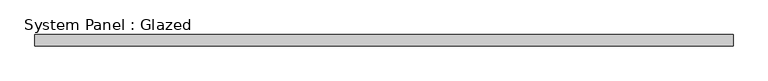
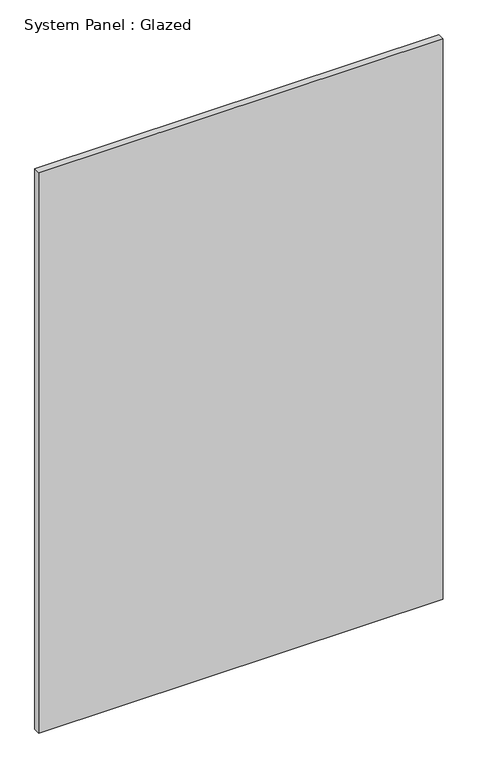
"""IFC4 building model written with IfcOpenShell, lengths in millimetres: plate geometry, System Panel : Glazed."""

from ifc_helpers import new_model, si_unit, origin, origin_with_axes, place, context, project, spatial, polyline, outline, extrude, source, transform, mapped, element, save


def system_panel_glazed_e50b416a(model_context):
    return source(origin(), model_context, "Body", "SweptSolid", [
        extrude(outline(polyline([(787.4, 19.05), (-787.4, 19.05), (-787.4, 44.45), (787.4, 44.45), (787.4, 19.05)])), origin_with_axes(), (0.0, 0.0, 1.0), 2306.7380434),
    ])


if __name__ == "__main__":
    model = new_model("IFC4")
    model_context = context("Model", 3, world=origin())
    ifc_project = project(units=[si_unit("LENGTHUNIT", "METRE", prefix="MILLI")], contexts=[model_context])
    site = spatial("IfcSite", under=ifc_project)
    building = spatial("IfcBuilding", under=site)
    placement = place(None, origin())
    system_panel_glazed_shape = system_panel_glazed_e50b416a(model_context)
    element("IfcPlate", 1, ObjectType="System Panel : Glazed", at=placement, inside=building, context=model_context, shape_type="MappedRepresentation", body=[
        mapped(system_panel_glazed_shape, transform((0.0, 0.0, 0.0), x_axis=(1.0, 0.0, 0.0), y_axis=(0.0, 1.0, 0.0), z_axis=(0.0, 0.0, 1.0))),
    ])
    save(model, "model.ifc")

# Revit data of these elements
# Type "System Panel : Glazed"
#   Construction Type Id = "GSP4R"
#   Analytic Construction = "1/8 in Pilkington single glazing"
#   Visual Light Transmittance = 0.9
#   Solar Heat Gain Coefficient = 0.86
#   Heat Transfer Coefficient (U) = 1.18115 BTU/(h·ft²·°F)
# Element 1 (IfcPlate, "System Panel : Glazed")
#   Materials on its faces: "Glass"
# Materials
#   "Glass": class "Glass", colour RGB 0 128 192, transparency 0.75, Description = "Soda Lime Glass", Cost = 0
